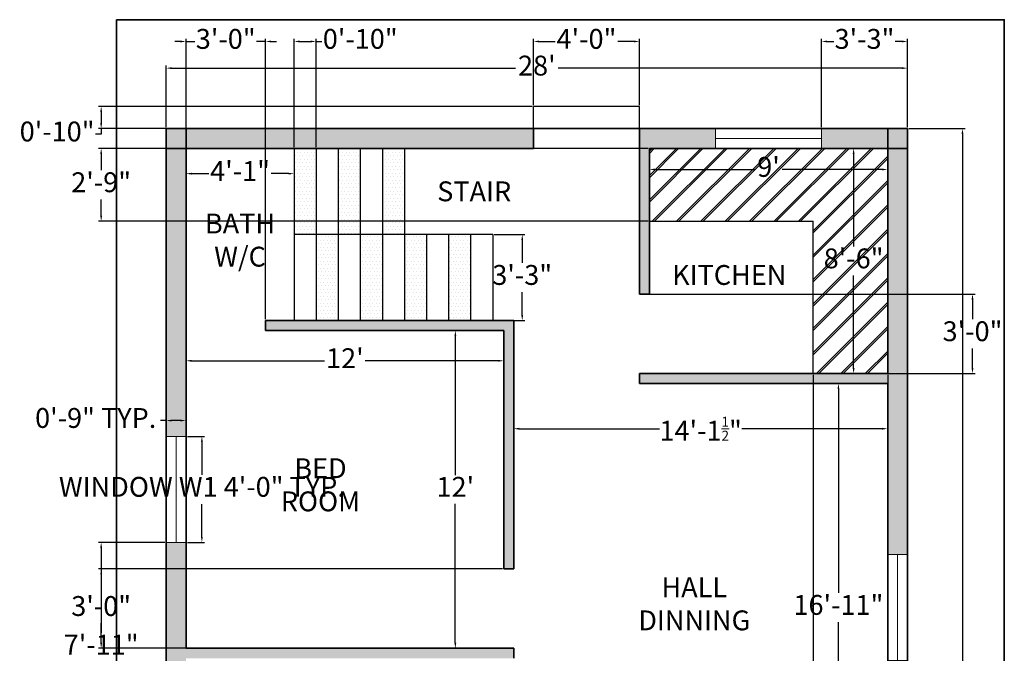
# Model space of a CAD drawing. Units: inches. Extents: x 4987 to 5457, y 8145 to 8785.
# Tile 3 of 3: x 4987 to 5434, y 8498 to 8785. Entities that reach past the tile are written whole.
import ezdxf

# ---------------------------------------------------------------- set-up
doc = ezdxf.new("R2010")
doc.units = ezdxf.units.IN
for name, color, linetype, lineweight in [('A-ANNO-DIMS', 2, 'Continuous', 18), ('A-ANNO-TTLB', 7, 'Continuous', 35), ('A-AREA-IDEN', 240, 'Continuous', 25), ('A-COLS', 7, 'Continuous', 35), ('A-COLS-PATT', 7, 'Continuous', 13), ('A-FLOR-FIXT', 8, 'Continuous', 25), ('A-FLOR-PATT', 8, 'Continuous', 13), ('A-FLOR-STRS', 7, 'Continuous', 25), ('A-GLAZ', 4, 'Continuous', 18), ('A-WALL', 7, 'Continuous', 35)]:
    doc.layers.add(name, color=color, linetype=linetype, lineweight=lineweight)
doc.layers.add('A-FIXT-PATT', color=67, linetype='Continuous', lineweight=13, true_color=0x727430)
doc.layers.add('A-WALL-PATT', color=67, linetype='Continuous', lineweight=13, true_color=0x727430)
doc.styles.get("Standard").update_dxf_attribs({"font": 'arial.ttf'})
doc.dimstyles.new('ISO-25', dxfattribs={"dimtxt": 9, "dimasz": 2.5, "dimexe": 1.25, "dimexo": 0.625, "dimgap": 2, "dimtad": 0, "dimtih": 1, "dimtoh": 1, "dimdec": 1, "dimlunit": 4, "dimtxsty": 'Standard', "dimcen": 2.5, "dimadec": 0, "dimazin": 0, "dimtfac": 0.5, "dimtdec": 1, "dimtmove": 0, "dimatfit": 3, "dimfxl": 1, "dimarcsym": 0})

# ---------------------------------------------------------------- blocks, each defined once
blk = doc.blocks.new('*D1')
at = {"layer": 'A-ANNO-DIMS', "color": 0, "lineweight": -2, "transparency": 16777216}
for p, q in [((5272.84, 8717.82), (5272.84, 8718.44)), ((5275.34, 8717.19), (5320.7, 8717.19)), ((5378.34, 8717.19), (5332.98, 8717.19)), ((5380.84, 8717.82), (5380.84, 8718.44))]:
    blk.add_line(p, q, dxfattribs=at)
at = {"layer": 'A-ANNO-DIMS', "color": 0, "transparency": 16777216}
for points in [[(5275.34, 8717.61), (5275.34, 8716.78), (5272.84, 8717.19)], [(5378.34, 8717.61), (5378.34, 8716.78), (5380.84, 8717.19)]]:
    blk.add_solid(points, dxfattribs=at)
at = {"layer": 'Defpoints', "color": 0, "transparency": 16777216}
for p in [(5272.84, 8717.19), (5380.84, 8717.19), (5380.84, 8717.19)]:
    blk.add_point(p, dxfattribs=at)
at = {"layer": 'A-ANNO-DIMS', "color": 0, "transparency": 16777216, "insert": (5326.84, 8717.19), "char_height": 9, "attachment_point": 5}
blk.add_mtext("9'", dxfattribs=at)
blk = doc.blocks.new('*D2')
at = {"layer": 'A-ANNO-DIMS', "color": 0, "lineweight": -2, "transparency": 16777216}
for p, q in [((5380.22, 8726.74), (5364.15, 8726.74)), ((5365.4, 8724.24), (5365.4, 8682.33)), ((5365.4, 8627.24), (5365.4, 8669.14)), ((5380.22, 8624.74), (5364.15, 8624.74))]:
    blk.add_line(p, q, dxfattribs=at)
at = {"layer": 'A-ANNO-DIMS', "color": 0, "transparency": 16777216}
for points in [[(5364.99, 8724.24), (5365.82, 8724.24), (5365.4, 8726.74)], [(5364.99, 8627.24), (5365.82, 8627.24), (5365.4, 8624.74)]]:
    blk.add_solid(points, dxfattribs=at)
at = {"layer": 'Defpoints', "color": 0, "transparency": 16777216}
for p in [(5365.4, 8726.74), (5380.84, 8726.74), (5380.84, 8624.74)]:
    blk.add_point(p, dxfattribs=at)
at = {"layer": 'A-ANNO-DIMS', "color": 0, "transparency": 16777216, "insert": (5365.4, 8675.74), "char_height": 9, "attachment_point": 5}
blk.add_mtext('8\'-6"', dxfattribs=at)
blk = doc.blocks.new('*D3')
at = {"layer": 'A-ANNO-DIMS', "color": 0, "lineweight": -2, "transparency": 16777216}
for p, q in [((5380.22, 8620.24), (5357.27, 8620.24)), ((5358.52, 8617.74), (5358.52, 8525.33)), ((5358.52, 8419.74), (5358.52, 8512.14)), ((5380.22, 8417.24), (5357.27, 8417.24))]:
    blk.add_line(p, q, dxfattribs=at)
at = {"layer": 'A-ANNO-DIMS', "color": 0, "transparency": 16777216}
for points in [[(5358.11, 8617.74), (5358.94, 8617.74), (5358.52, 8620.24)], [(5358.11, 8419.74), (5358.94, 8419.74), (5358.52, 8417.24)]]:
    blk.add_solid(points, dxfattribs=at)
at = {"layer": 'Defpoints', "color": 0, "transparency": 16777216}
for p in [(5380.84, 8620.24), (5358.52, 8417.24), (5380.84, 8417.24)]:
    blk.add_point(p, dxfattribs=at)
at = {"layer": 'A-ANNO-DIMS', "color": 0, "transparency": 16777216, "insert": (5358.52, 8518.74), "char_height": 9, "attachment_point": 5}
blk.add_mtext('16\'-11"', dxfattribs=at)
blk = doc.blocks.new('*D4')
at = {"layer": 'A-ANNO-DIMS', "color": 0, "lineweight": -2, "transparency": 16777216}
for p, q in [((5211.34, 8619.61), (5211.34, 8598.5)), ((5380.84, 8619.61), (5380.84, 8598.5)), ((5213.84, 8599.75), (5277.41, 8599.75)), ((5378.34, 8599.75), (5314.77, 8599.75))]:
    blk.add_line(p, q, dxfattribs=at)
at = {"layer": 'A-ANNO-DIMS', "color": 0, "transparency": 16777216}
for points in [[(5213.84, 8600.16), (5213.84, 8599.33), (5211.34, 8599.75)], [(5378.34, 8600.16), (5378.34, 8599.33), (5380.84, 8599.75)]]:
    blk.add_solid(points, dxfattribs=at)
at = {"layer": 'Defpoints', "color": 0, "transparency": 16777216}
for p in [(5211.34, 8620.24), (5380.84, 8620.24), (5211.34, 8599.75)]:
    blk.add_point(p, dxfattribs=at)
at = {"layer": 'A-ANNO-DIMS', "color": 0, "transparency": 16777216, "insert": (5296.09, 8599.75), "char_height": 9, "attachment_point": 5}
blk.add_mtext('14\'-1{\\H0.5x;\\S1/2;}"', dxfattribs=at)
blk = doc.blocks.new('*D5')
at = {"layer": 'A-ANNO-DIMS', "color": 0, "lineweight": -2, "transparency": 16777216}
for p, q in [((5202.47, 8687.74), (5216.47, 8687.74)), ((5215.22, 8685.24), (5215.22, 8674.83)), ((5215.22, 8651.24), (5215.22, 8661.64)), ((5202.47, 8648.74), (5216.47, 8648.74))]:
    blk.add_line(p, q, dxfattribs=at)
at = {"layer": 'A-ANNO-DIMS', "color": 0, "transparency": 16777216}
for points in [[(5214.8, 8685.24), (5215.64, 8685.24), (5215.22, 8687.74)], [(5214.8, 8651.24), (5215.64, 8651.24), (5215.22, 8648.74)]]:
    blk.add_solid(points, dxfattribs=at)
at = {"layer": 'Defpoints', "color": 0, "transparency": 16777216}
for p in [(5201.84, 8687.74), (5215.22, 8687.74), (5201.84, 8648.74)]:
    blk.add_point(p, dxfattribs=at)
at = {"layer": 'A-ANNO-DIMS', "color": 0, "transparency": 16777216, "insert": (5215.22, 8668.24), "char_height": 9, "attachment_point": 5}
blk.add_mtext('3\'-3"', dxfattribs=at)
blk = doc.blocks.new('*D6')
at = {"layer": 'A-ANNO-DIMS', "color": 0, "lineweight": -2, "transparency": 16777216}
for p, q in [((5062.84, 8726.11), (5062.84, 8714.05)), ((5111.84, 8726.11), (5111.84, 8714.05)), ((5065.34, 8715.3), (5073.2, 8715.3)), ((5109.34, 8715.3), (5101.48, 8715.3))]:
    blk.add_line(p, q, dxfattribs=at)
at = {"layer": 'A-ANNO-DIMS', "color": 0, "transparency": 16777216}
for points in [[(5065.34, 8715.71), (5065.34, 8714.88), (5062.84, 8715.3)], [(5109.34, 8715.71), (5109.34, 8714.88), (5111.84, 8715.3)]]:
    blk.add_solid(points, dxfattribs=at)
at = {"layer": 'Defpoints', "color": 0, "transparency": 16777216}
for p in [(5062.84, 8726.74), (5111.84, 8726.74), (5062.84, 8715.3)]:
    blk.add_point(p, dxfattribs=at)
at = {"layer": 'A-ANNO-DIMS', "color": 0, "transparency": 16777216, "insert": (5087.34, 8715.3), "char_height": 9, "attachment_point": 5}
blk.add_mtext('4\'-1"', dxfattribs=at)
blk = doc.blocks.new('*D7')
at = {"layer": 'A-ANNO-DIMS', "color": 0, "lineweight": -2, "transparency": 16777216}
for p, q in [((5062.84, 8643.61), (5062.84, 8629.26)), ((5206.84, 8643.61), (5206.84, 8629.26)), ((5065.34, 8630.51), (5125.63, 8630.51)), ((5204.34, 8630.51), (5144.05, 8630.51))]:
    blk.add_line(p, q, dxfattribs=at)
at = {"layer": 'A-ANNO-DIMS', "color": 0, "transparency": 16777216}
for points in [[(5065.34, 8630.93), (5065.34, 8630.1), (5062.84, 8630.51)], [(5204.34, 8630.93), (5204.34, 8630.1), (5206.84, 8630.51)]]:
    blk.add_solid(points, dxfattribs=at)
at = {"layer": 'Defpoints', "color": 0, "transparency": 16777216}
for p in [(5062.84, 8644.24), (5206.84, 8644.24), (5062.84, 8630.51)]:
    blk.add_point(p, dxfattribs=at)
at = {"layer": 'A-ANNO-DIMS', "color": 0, "transparency": 16777216, "insert": (5134.84, 8630.51), "char_height": 9, "attachment_point": 5}
blk.add_mtext("12'", dxfattribs=at)
blk = doc.blocks.new('*D8')
at = {"layer": 'A-ANNO-DIMS', "color": 0, "lineweight": -2, "transparency": 16777216}
for p, q in [((5185.53, 8644.24), (5186.15, 8644.24)), ((5184.9, 8641.74), (5184.9, 8578.75)), ((5184.9, 8502.74), (5184.9, 8565.72)), ((5185.53, 8500.24), (5186.15, 8500.24))]:
    blk.add_line(p, q, dxfattribs=at)
at = {"layer": 'A-ANNO-DIMS', "color": 0, "transparency": 16777216}
for points in [[(5184.49, 8641.74), (5185.32, 8641.74), (5184.9, 8644.24)], [(5184.49, 8502.74), (5185.32, 8502.74), (5184.9, 8500.24)]]:
    blk.add_solid(points, dxfattribs=at)
at = {"layer": 'Defpoints', "color": 0, "transparency": 16777216}
for p in [(5184.9, 8644.24), (5184.9, 8644.24), (5184.9, 8500.24)]:
    blk.add_point(p, dxfattribs=at)
at = {"layer": 'A-ANNO-DIMS', "color": 0, "transparency": 16777216, "insert": (5184.9, 8572.24), "char_height": 9, "attachment_point": 5}
blk.add_mtext("12'", dxfattribs=at)
blk = doc.blocks.new('*D19')
at = {"layer": 'A-ANNO-DIMS', "color": 0, "lineweight": -2, "transparency": 16777216}
for p, q in [((5390.47, 8735.74), (5415.98, 8735.74)), ((5414.73, 8733.24), (5414.73, 8478.24)), ((5414.73, 8210.24), (5414.73, 8465.24)), ((5390.47, 8207.74), (5415.98, 8207.74))]:
    blk.add_line(p, q, dxfattribs=at)
at = {"layer": 'A-ANNO-DIMS', "color": 0, "transparency": 16777216}
for points in [[(5414.31, 8733.24), (5415.15, 8733.24), (5414.73, 8735.74)], [(5414.31, 8210.24), (5415.15, 8210.24), (5414.73, 8207.74)]]:
    blk.add_solid(points, dxfattribs=at)
at = {"layer": 'Defpoints', "color": 0, "transparency": 16777216}
for p in [(5389.84, 8735.74), (5389.84, 8207.74), (5414.73, 8207.74)]:
    blk.add_point(p, dxfattribs=at)
at = {"layer": 'A-ANNO-DIMS', "color": 0, "transparency": 16777216, "insert": (5414.73, 8471.74), "char_height": 9, "attachment_point": 5}
blk.add_mtext("44'", dxfattribs=at)
blk = doc.blocks.new('*D20')
at = {"layer": 'A-ANNO-DIMS', "color": 0, "lineweight": -2, "transparency": 16777216}
for p, q in [((5053.84, 8736.36), (5053.84, 8764.35)), ((5389.84, 8736.36), (5389.84, 8764.35)), ((5056.34, 8763.1), (5212.13, 8763.1)), ((5387.34, 8763.1), (5231.55, 8763.1))]:
    blk.add_line(p, q, dxfattribs=at)
at = {"layer": 'A-ANNO-DIMS', "color": 0, "transparency": 16777216}
for points in [[(5056.34, 8763.52), (5056.34, 8762.68), (5053.84, 8763.1)], [(5387.34, 8763.52), (5387.34, 8762.68), (5389.84, 8763.1)]]:
    blk.add_solid(points, dxfattribs=at)
at = {"layer": 'Defpoints', "color": 0, "transparency": 16777216}
for p in [(5389.84, 8763.1), (5053.84, 8735.74), (5389.84, 8735.74)]:
    blk.add_point(p, dxfattribs=at)
at = {"layer": 'A-ANNO-DIMS', "color": 0, "transparency": 16777216, "insert": (5221.84, 8763.1), "char_height": 9, "attachment_point": 5}
blk.add_mtext("28'", dxfattribs=at)
blk = doc.blocks.new('WIN-48IN')
for p, q in [((0, 0), (0, 9)), ((48, 0), (48, 9)), ((0, 4.5), (48, 4.5))]:
    blk.add_line(p, q)
blk = doc.blocks.new('COL-CORNER-9IN')
for q in [(0, 0), (9, 9)]:
    blk.add_line((0, 9), q)
blk = doc.blocks.new('*D24')
at = {"layer": 'A-ANNO-DIMS', "color": 0, "lineweight": -2, "transparency": 16777216}
for p, q in [((5063.47, 8596.24), (5071.29, 8596.24)), ((5070.04, 8593.74), (5070.04, 8578.89)), ((5070.04, 8550.74), (5070.04, 8565.58)), ((5063.47, 8548.24), (5071.29, 8548.24))]:
    blk.add_line(p, q, dxfattribs=at)
at = {"layer": 'A-ANNO-DIMS', "color": 0, "transparency": 16777216}
for points in [[(5069.62, 8593.74), (5070.46, 8593.74), (5070.04, 8596.24)], [(5069.62, 8550.74), (5070.46, 8550.74), (5070.04, 8548.24)]]:
    blk.add_solid(points, dxfattribs=at)
at = {"layer": 'Defpoints', "color": 0, "transparency": 16777216}
for p in [(5062.84, 8596.24), (5070.04, 8596.24), (5062.84, 8548.24)]:
    blk.add_point(p, dxfattribs=at)
at = {"layer": 'A-ANNO-DIMS', "color": 0, "transparency": 16777216, "insert": (5070.04, 8572.24), "char_height": 9, "attachment_point": 5}
blk.add_mtext('WINDOW W1 4\'-0" TYP.', dxfattribs=at)
blk = doc.blocks.new('*D25')
at = {"layer": 'A-ANNO-DIMS', "color": 0, "lineweight": -2, "transparency": 16777216}
for p, q in [((5053.84, 8596.86), (5053.84, 8604.69)), ((5062.84, 8596.86), (5062.84, 8604.69)), ((5053.84, 8603.44), (5051.34, 8603.44)), ((5060.34, 8603.44), (5056.34, 8603.44))]:
    blk.add_line(p, q, dxfattribs=at)
at = {"layer": 'A-ANNO-DIMS', "color": 0, "transparency": 16777216}
for points in [[(5056.34, 8603.85), (5056.34, 8603.02), (5053.84, 8603.44)], [(5060.34, 8603.85), (5060.34, 8603.02), (5062.84, 8603.44)]]:
    blk.add_solid(points, dxfattribs=at)
at = {"layer": 'Defpoints', "color": 0, "transparency": 16777216}
for p in [(5053.84, 8603.44), (5053.84, 8596.24), (5062.84, 8596.24)]:
    blk.add_point(p, dxfattribs=at)
at = {"layer": 'A-ANNO-DIMS', "color": 0, "transparency": 16777216, "insert": (5021.91, 8603.44), "char_height": 9, "attachment_point": 5}
blk.add_mtext('0\'-9" TYP.', dxfattribs=at)
blk = doc.blocks.new('*D32')
at = {"layer": 'A-ANNO-DIMS', "color": 0, "lineweight": -2, "transparency": 16777216}
for p, q in [((5053.22, 8548.24), (5023.14, 8548.24)), ((5024.39, 8545.74), (5024.39, 8507.25)), ((5024.39, 8455.74), (5024.39, 8494.22)), ((5053.22, 8453.24), (5023.14, 8453.24))]:
    blk.add_line(p, q, dxfattribs=at)
at = {"layer": 'A-ANNO-DIMS', "color": 0, "transparency": 16777216}
for points in [[(5023.97, 8545.74), (5024.81, 8545.74), (5024.39, 8548.24)], [(5023.97, 8455.74), (5024.81, 8455.74), (5024.39, 8453.24)]]:
    blk.add_solid(points, dxfattribs=at)
at = {"layer": 'Defpoints', "color": 0, "transparency": 16777216}
for p in [(5024.39, 8548.24), (5053.84, 8548.24), (5053.84, 8453.24)]:
    blk.add_point(p, dxfattribs=at)
at = {"layer": 'A-ANNO-DIMS', "color": 0, "transparency": 16777216, "insert": (5024.39, 8500.74), "char_height": 9, "attachment_point": 5}
blk.add_mtext('7\'-11"', dxfattribs=at)
blk = doc.blocks.new('*D36')
at = {"layer": 'A-ANNO-DIMS', "color": 0, "lineweight": -2, "transparency": 16777216}
for p, q in [((5350.84, 8736.36), (5350.84, 8776.44)), ((5353.34, 8775.19), (5356.38, 8775.19)), ((5387.34, 8775.19), (5384.3, 8775.19)), ((5389.84, 8736.36), (5389.84, 8776.44))]:
    blk.add_line(p, q, dxfattribs=at)
at = {"layer": 'A-ANNO-DIMS', "color": 0, "transparency": 16777216}
for points in [[(5353.34, 8775.6), (5353.34, 8774.77), (5350.84, 8775.19)], [(5387.34, 8775.6), (5387.34, 8774.77), (5389.84, 8775.19)]]:
    blk.add_solid(points, dxfattribs=at)
at = {"layer": 'Defpoints', "color": 0, "transparency": 16777216}
for p in [(5389.84, 8775.19), (5350.84, 8735.74), (5389.84, 8735.74)]:
    blk.add_point(p, dxfattribs=at)
at = {"layer": 'A-ANNO-DIMS', "color": 0, "transparency": 16777216, "insert": (5370.34, 8775.19), "char_height": 9, "attachment_point": 5}
blk.add_mtext('3\'-3"', dxfattribs=at)
blk = doc.blocks.new('*D39')
at = {"layer": 'A-ANNO-DIMS', "color": 0, "lineweight": -2, "transparency": 16777216}
for p, q in [((5220.34, 8746.36), (5220.34, 8776.44)), ((5222.84, 8775.19), (5230.2, 8775.19)), ((5265.84, 8775.19), (5258.48, 8775.19)), ((5268.34, 8746.36), (5268.34, 8776.44))]:
    blk.add_line(p, q, dxfattribs=at)
at = {"layer": 'A-ANNO-DIMS', "color": 0, "transparency": 16777216}
for points in [[(5222.84, 8775.6), (5222.84, 8774.77), (5220.34, 8775.19)], [(5265.84, 8775.6), (5265.84, 8774.77), (5268.34, 8775.19)]]:
    blk.add_solid(points, dxfattribs=at)
at = {"layer": 'Defpoints', "color": 0, "transparency": 16777216}
for p in [(5268.34, 8775.19), (5220.34, 8745.74), (5268.34, 8745.74)]:
    blk.add_point(p, dxfattribs=at)
at = {"layer": 'A-ANNO-DIMS', "color": 0, "transparency": 16777216, "insert": (5244.34, 8775.19), "char_height": 9, "attachment_point": 5}
blk.add_mtext('4\'-0"', dxfattribs=at)
blk = doc.blocks.new('*D40')
at = {"layer": 'A-ANNO-DIMS', "color": 0, "lineweight": -2, "transparency": 16777216}
for p, q in [((5219.72, 8745.74), (5023.14, 8745.74)), ((5024.39, 8743.24), (5024.39, 8738.24)), ((5024.39, 8733.24), (5021.89, 8733.24)), ((5219.72, 8735.74), (5023.14, 8735.74)), ((5024.39, 8735.74), (5024.39, 8733.24))]:
    blk.add_line(p, q, dxfattribs=at)
at = {"layer": 'A-ANNO-DIMS', "color": 0, "transparency": 16777216}
for points in [[(5023.97, 8743.24), (5024.81, 8743.24), (5024.39, 8745.74)], [(5023.97, 8738.24), (5024.81, 8738.24), (5024.39, 8735.74)]]:
    blk.add_solid(points, dxfattribs=at)
at = {"layer": 'Defpoints', "color": 0, "transparency": 16777216}
for p in [(5220.34, 8745.74), (5024.39, 8735.74), (5220.34, 8735.74)]:
    blk.add_point(p, dxfattribs=at)
at = {"layer": 'A-ANNO-DIMS', "color": 0, "transparency": 16777216, "insert": (5004.43, 8733.24), "char_height": 9, "attachment_point": 5}
blk.add_mtext('0\'-10"', dxfattribs=at)
blk = doc.blocks.new('*D41')
at = {"layer": 'A-ANNO-DIMS', "color": 0, "lineweight": -2, "transparency": 16777216}
for p, q in [((5111.84, 8727.36), (5111.84, 8776.44)), ((5114.34, 8775.19), (5119.34, 8775.19)), ((5121.84, 8727.36), (5121.84, 8776.44)), ((5121.84, 8775.19), (5124.34, 8775.19))]:
    blk.add_line(p, q, dxfattribs=at)
at = {"layer": 'A-ANNO-DIMS', "color": 0, "transparency": 16777216}
for points in [[(5114.34, 8775.6), (5114.34, 8774.77), (5111.84, 8775.19)], [(5119.34, 8775.6), (5119.34, 8774.77), (5121.84, 8775.19)]]:
    blk.add_solid(points, dxfattribs=at)
at = {"layer": 'Defpoints', "color": 0, "transparency": 16777216}
for p in [(5121.84, 8775.19), (5111.84, 8726.74), (5121.84, 8726.74)]:
    blk.add_point(p, dxfattribs=at)
at = {"layer": 'A-ANNO-DIMS', "color": 0, "transparency": 16777216, "insert": (5141.8, 8775.19), "char_height": 9, "attachment_point": 5}
blk.add_mtext('0\'-10"', dxfattribs=at)
blk = doc.blocks.new('*D42')
at = {"layer": 'A-ANNO-DIMS', "color": 0, "lineweight": -2, "transparency": 16777216}
for p, q in [((5347.07, 8624.11), (5347.07, 8157.04)), ((5380.84, 8624.11), (5380.84, 8157.04)), ((5349.57, 8158.29), (5378.34, 8158.29)), ((5380.84, 8158.29), (5383.34, 8158.29))]:
    blk.add_line(p, q, dxfattribs=at)
at = {"layer": 'A-ANNO-DIMS', "color": 0, "transparency": 16777216}
for points in [[(5349.57, 8158.7), (5349.57, 8157.87), (5347.07, 8158.29)], [(5378.34, 8158.7), (5378.34, 8157.87), (5380.84, 8158.29)]]:
    blk.add_solid(points, dxfattribs=at)
at = {"layer": 'Defpoints', "color": 0, "transparency": 16777216}
for p in [(5347.07, 8624.74), (5380.84, 8624.74), (5380.84, 8158.29)]:
    blk.add_point(p, dxfattribs=at)
at = {"layer": 'A-ANNO-DIMS', "color": 0, "transparency": 16777216, "insert": (5400.88, 8158.29), "char_height": 9, "attachment_point": 5}
blk.add_mtext('2\'-10"', dxfattribs=at)
blk = doc.blocks.new('*D43')
at = {"layer": 'A-ANNO-DIMS', "color": 0, "lineweight": -2, "transparency": 16777216}
for p, q in [((5272.22, 8726.74), (5023.14, 8726.74)), ((5024.39, 8724.24), (5024.39, 8716.83)), ((5024.39, 8696.24), (5024.39, 8703.64)), ((5272.22, 8693.74), (5023.14, 8693.74))]:
    blk.add_line(p, q, dxfattribs=at)
at = {"layer": 'A-ANNO-DIMS', "color": 0, "transparency": 16777216}
for points in [[(5023.97, 8724.24), (5024.81, 8724.24), (5024.39, 8726.74)], [(5023.97, 8696.24), (5024.81, 8696.24), (5024.39, 8693.74)]]:
    blk.add_solid(points, dxfattribs=at)
at = {"layer": 'Defpoints', "color": 0, "transparency": 16777216}
for p in [(5024.39, 8726.74), (5272.84, 8726.74), (5272.84, 8693.74)]:
    blk.add_point(p, dxfattribs=at)
at = {"layer": 'A-ANNO-DIMS', "color": 0, "transparency": 16777216, "insert": (5024.39, 8710.24), "char_height": 9, "attachment_point": 5}
blk.add_mtext('2\'-9"', dxfattribs=at)
blk = doc.blocks.new('*D44')
at = {"layer": 'A-ANNO-DIMS', "color": 0, "lineweight": -2, "transparency": 16777216}
for p, q in [((5268.97, 8660.74), (5420.54, 8660.74)), ((5419.29, 8658.24), (5419.29, 8649.33)), ((5419.29, 8627.24), (5419.29, 8636.14)), ((5268.97, 8624.74), (5420.54, 8624.74))]:
    blk.add_line(p, q, dxfattribs=at)
at = {"layer": 'A-ANNO-DIMS', "color": 0, "transparency": 16777216}
for points in [[(5418.87, 8658.24), (5419.71, 8658.24), (5419.29, 8660.74)], [(5418.87, 8627.24), (5419.71, 8627.24), (5419.29, 8624.74)]]:
    blk.add_solid(points, dxfattribs=at)
at = {"layer": 'Defpoints', "color": 0, "transparency": 16777216}
for p in [(5268.34, 8660.74), (5419.29, 8660.74), (5268.34, 8624.74)]:
    blk.add_point(p, dxfattribs=at)
at = {"layer": 'A-ANNO-DIMS', "color": 0, "transparency": 16777216, "insert": (5419.29, 8642.74), "char_height": 9, "attachment_point": 5}
blk.add_mtext('3\'-0"', dxfattribs=at)
blk = doc.blocks.new('*D45')
at = {"layer": 'A-ANNO-DIMS', "color": 0, "lineweight": -2, "transparency": 16777216}
for p, q in [((5206.22, 8536.24), (5023.14, 8536.24)), ((5024.39, 8533.74), (5024.39, 8524.83)), ((5024.39, 8502.74), (5024.39, 8511.64)), ((5206.22, 8500.24), (5023.14, 8500.24))]:
    blk.add_line(p, q, dxfattribs=at)
at = {"layer": 'A-ANNO-DIMS', "color": 0, "transparency": 16777216}
for points in [[(5023.97, 8533.74), (5024.81, 8533.74), (5024.39, 8536.24)], [(5023.97, 8502.74), (5024.81, 8502.74), (5024.39, 8500.24)]]:
    blk.add_solid(points, dxfattribs=at)
at = {"layer": 'Defpoints', "color": 0, "transparency": 16777216}
for p in [(5024.39, 8536.24), (5206.84, 8536.24), (5206.84, 8500.24)]:
    blk.add_point(p, dxfattribs=at)
at = {"layer": 'A-ANNO-DIMS', "color": 0, "transparency": 16777216, "insert": (5024.39, 8518.24), "char_height": 9, "attachment_point": 5}
blk.add_mtext('3\'-0"', dxfattribs=at)
blk = doc.blocks.new('*D50')
at = {"layer": 'A-ANNO-DIMS', "color": 0, "lineweight": -2, "transparency": 16777216}
for p, q in [((5060.34, 8775.19), (5057.84, 8775.19)), ((5062.84, 8649.36), (5062.84, 8776.44)), ((5062.84, 8775.19), (5066.88, 8775.19)), ((5098.84, 8775.19), (5094.8, 8775.19)), ((5098.84, 8649.36), (5098.84, 8776.44)), ((5101.34, 8775.19), (5103.84, 8775.19))]:
    blk.add_line(p, q, dxfattribs=at)
at = {"layer": 'A-ANNO-DIMS', "color": 0, "transparency": 16777216}
for points in [[(5060.34, 8775.6), (5060.34, 8774.77), (5062.84, 8775.19)], [(5101.34, 8775.6), (5101.34, 8774.77), (5098.84, 8775.19)]]:
    blk.add_solid(points, dxfattribs=at)
at = {"layer": 'Defpoints', "color": 0, "transparency": 16777216}
for p in [(5098.84, 8775.19), (5062.84, 8648.74), (5098.84, 8648.74)]:
    blk.add_point(p, dxfattribs=at)
at = {"layer": 'A-ANNO-DIMS', "color": 0, "transparency": 16777216, "insert": (5080.84, 8775.19), "char_height": 9, "attachment_point": 5}
blk.add_mtext('3\'-0"', dxfattribs=at)

msp = doc.modelspace()

# ---------------------------------------------------------------- hatches: boundary and pattern name
at = {"layer": 'A-COLS-PATT'}
h = msp.add_hatch(color=256, dxfattribs=at)
h.dxf.hatch_style = 1
h.paths.add_polyline_path([(5062.84, 8735.74), (5053.84, 8735.74), (5053.84, 8726.74), (5062.84, 8726.74)])
h.paths.add_polyline_path([(5389.84, 8735.74), (5380.84, 8735.74), (5380.84, 8726.74), (5389.84, 8726.74)])
h.paths.add_polyline_path([(5389.84, 8216.74), (5380.84, 8216.74), (5380.84, 8207.74), (5389.84, 8207.74)])
h.paths.add_polyline_path([(5062.84, 8216.74), (5053.84, 8216.74), (5053.84, 8207.74), (5062.84, 8207.74)])
at = {"layer": 'A-FIXT-PATT'}
h = msp.add_hatch(dxfattribs=at)
h.set_pattern_fill('JIS_LC_8A', color=256)
h.paths.add_polyline_path([(5380.84, 8726.74), (5272.84, 8726.74), (5272.84, 8693.74), (5347.07, 8693.74), (5347.07, 8624.74), (5380.84, 8624.74)])
at = {"layer": 'A-FLOR-PATT'}
h = msp.add_hatch(dxfattribs=at)
h.set_pattern_fill('DOTS', color=256)
h.paths.add_polyline_path([(5121.84, 8726.74), (5111.84, 8726.74), (5111.84, 8687.74), (5121.84, 8687.74)])
h.paths.add_polyline_path([(5141.84, 8726.74), (5131.84, 8726.74), (5131.84, 8687.74), (5141.84, 8687.74)])
h.paths.add_polyline_path([(5161.84, 8726.74), (5151.84, 8726.74), (5151.84, 8687.74), (5161.84, 8687.74)])
h.paths.add_polyline_path([(5131.84, 8687.74), (5121.84, 8687.74), (5121.84, 8648.74), (5131.84, 8648.74)])
h.paths.add_polyline_path([(5151.84, 8687.74), (5141.84, 8687.74), (5141.84, 8648.74), (5151.84, 8648.74)])
h.paths.add_polyline_path([(5171.84, 8687.74), (5161.84, 8687.74), (5161.84, 8648.74), (5171.84, 8648.74)])
h.paths.add_polyline_path([(5191.84, 8687.74), (5181.84, 8687.74), (5181.84, 8648.74), (5191.84, 8648.74)])
at = {"layer": 'A-WALL-PATT'}
h = msp.add_hatch(color=256, dxfattribs=at)
h.dxf.hatch_style = 1
h.paths.add_polyline_path([(5220.34, 8735.74), (5062.84, 8735.74), (5062.84, 8726.74), (5111.84, 8726.74), (5220.34, 8726.74)])
h.paths.add_polyline_path([(5062.84, 8548.24), (5053.84, 8548.24), (5053.84, 8453.24), (5062.84, 8453.24), (5062.84, 8495.74), (5206.84, 8495.74), (5211.34, 8495.74), (5211.34, 8500.24), (5206.84, 8500.24), (5062.84, 8500.24)])
h.paths.add_polyline_path([(5211.34, 8362.74), (5211.34, 8412.74), (5211.34, 8417.24), (5211.34, 8459.74), (5206.84, 8459.74), (5206.84, 8417.24), (5206.84, 8412.74), (5206.84, 8362.74), (5062.84, 8362.74), (5062.84, 8405.24), (5053.84, 8405.24), (5053.84, 8311.49), (5062.84, 8311.49), (5062.84, 8358.24), (5206.84, 8358.24), (5211.34, 8358.24)])
h.paths.add_polyline_path([(5062.84, 8263.49), (5053.84, 8263.49), (5053.84, 8216.74), (5062.84, 8216.74)])
h.paths.add_polyline_path([(5211.34, 8216.74), (5206.84, 8216.74), (5062.84, 8216.74), (5062.84, 8207.74), (5211.34, 8207.74)])
h.paths.add_polyline_path([(5380.84, 8216.74), (5271.34, 8216.74), (5271.34, 8207.74), (5380.84, 8207.74)])
h.paths.add_polyline_path([(5389.84, 8314.24), (5380.84, 8314.24), (5380.84, 8305.24), (5332.84, 8305.24), (5332.84, 8311.24), (5328.34, 8311.24), (5328.34, 8305.24), (5247.34, 8305.24), (5247.34, 8300.74), (5380.84, 8300.74), (5380.84, 8216.74), (5389.84, 8216.74)])
h.paths.add_polyline_path([(5389.84, 8370.24), (5380.84, 8370.24), (5380.84, 8351.74), (5328.34, 8351.74), (5320.84, 8351.74), (5320.84, 8347.24), (5328.34, 8347.24), (5332.84, 8347.24), (5380.84, 8347.24), (5380.84, 8338.24), (5389.84, 8338.24)])
h.paths.add_polyline_path([(5389.84, 8494.74), (5380.84, 8494.74), (5380.84, 8417.24), (5280.34, 8417.24), (5280.34, 8412.74), (5280.34, 8351.74), (5280.34, 8347.24), (5284.84, 8347.24), (5284.84, 8351.74), (5284.84, 8412.74), (5328.34, 8412.74), (5380.84, 8412.74), (5380.84, 8394.24), (5389.84, 8394.24)])
h.paths.add_polyline_path([(5389.84, 8726.74), (5380.84, 8726.74), (5380.84, 8624.74), (5272.84, 8624.74), (5268.34, 8624.74), (5268.34, 8620.24), (5380.84, 8620.24), (5380.84, 8542.74), (5389.84, 8542.74)])
h.paths.add_polyline_path([(5062.84, 8726.74), (5053.84, 8726.74), (5053.84, 8596.24), (5062.84, 8596.24), (5062.84, 8644.24), (5062.84, 8648.74)])
h.paths.add_polyline_path([(5302.84, 8735.74), (5268.34, 8735.74), (5268.34, 8726.74), (5268.34, 8660.74), (5272.84, 8660.74), (5272.84, 8726.74), (5302.84, 8726.74)])
h.paths.add_polyline_path([(5380.84, 8735.74), (5350.84, 8735.74), (5350.84, 8726.74), (5380.84, 8726.74)])
h.paths.add_polyline_path([(5211.34, 8648.74), (5206.84, 8648.74), (5098.84, 8648.74), (5098.84, 8644.24), (5206.84, 8644.24), (5206.84, 8624.74), (5206.84, 8536.24), (5211.34, 8536.24), (5211.34, 8620.24), (5211.34, 8624.74)])
h.paths.add_polyline_path([(5211.34, 8305.24), (5211.34, 8322.24), (5206.84, 8322.24), (5206.84, 8305.24), (5206.84, 8300.74), (5206.84, 8252.74), (5211.34, 8252.74), (5211.34, 8300.74)])

# ---------------------------------------------------------------- linework, layer by layer
at = {"layer": 'A-ANNO-TTLB'}
msp.add_lwpolyline([(5031.32, 8785.05), (5433.7, 8785.05), (5433.7, 8175.66), (5031.32, 8175.66)], close=True, dxfattribs=at)
at = {"layer": 'A-FLOR-FIXT'}
for p in [(5272.84, 8693.74), (5347.07, 8624.74)]:
    msp.add_line(p, (5347.07, 8693.74), dxfattribs=at)
at = {"layer": 'A-FLOR-STRS'}
for p, q in [((5220.34, 8735.74), (5220.34, 8745.74)), ((5268.34, 8745.74), (5220.34, 8745.74)), ((5268.34, 8735.74), (5268.34, 8745.74)), ((5111.84, 8726.74), (5111.84, 8648.74)), ((5121.84, 8726.74), (5121.84, 8648.74)), ((5131.84, 8726.74), (5131.84, 8648.74)), ((5141.84, 8726.74), (5141.84, 8648.74)), ((5151.84, 8726.74), (5151.84, 8648.74)), ((5161.84, 8726.74), (5161.84, 8648.74)), ((5201.84, 8687.74), (5111.84, 8687.74)), ((5171.84, 8687.74), (5171.84, 8648.74)), ((5181.84, 8687.74), (5181.84, 8648.74)), ((5191.84, 8687.74), (5191.84, 8648.74)), ((5201.84, 8687.74), (5201.84, 8648.74))]:
    msp.add_line(p, q, dxfattribs=at)
at = {"layer": 'A-WALL'}
for p, q in [((5053.84, 8735.74), (5389.84, 8735.74)), ((5053.84, 8207.74), (5053.84, 8735.74)), ((5220.34, 8726.74), (5220.34, 8735.74)), ((5268.34, 8726.74), (5268.34, 8735.74)), ((5389.84, 8735.74), (5389.84, 8207.74)), ((5062.84, 8726.74), (5220.34, 8726.74)), ((5062.84, 8648.74), (5062.84, 8726.74)), ((5062.84, 8726.74), (5111.84, 8726.74)), ((5268.34, 8726.74), (5268.34, 8660.74)), ((5272.84, 8726.74), (5272.84, 8660.74)), ((5272.84, 8726.74), (5380.84, 8726.74)), ((5380.84, 8726.74), (5380.84, 8624.74)), ((5272.84, 8660.74), (5268.34, 8660.74)), ((5062.84, 8648.74), (5062.84, 8644.24)), ((5206.84, 8648.74), (5098.84, 8648.74)), ((5098.84, 8648.74), (5098.84, 8644.24)), ((5206.84, 8648.74), (5211.34, 8648.74)), ((5211.34, 8624.74), (5211.34, 8648.74)), ((5062.84, 8500.24), (5062.84, 8644.24)), ((5206.84, 8644.24), (5098.84, 8644.24)), ((5206.84, 8644.24), (5206.84, 8624.74)), ((5206.84, 8624.74), (5206.84, 8536.24)), ((5211.34, 8624.74), (5211.34, 8620.24)), ((5268.34, 8624.74), (5268.34, 8620.24)), ((5272.84, 8624.74), (5268.34, 8624.74)), ((5380.84, 8624.74), (5272.84, 8624.74)), ((5211.34, 8620.24), (5211.34, 8536.24)), ((5380.84, 8620.24), (5268.34, 8620.24)), ((5380.84, 8620.24), (5380.84, 8417.24)), ((5206.84, 8536.24), (5211.34, 8536.24)), ((5206.84, 8500.24), (5062.84, 8500.24)), ((5206.84, 8500.24), (5211.34, 8500.24)), ((5211.34, 8500.24), (5211.34, 8495.74))]:
    msp.add_line(p, q, dxfattribs=at)

# ---------------------------------------------------------------- block references
at = {"layer": 'A-COLS'}
for p, rotation in [((5062.84, 8735.74), 180), ((5389.84, 8726.73), 89.9999999999884)]:
    msp.add_blockref('COL-CORNER-9IN', p, dxfattribs=dict(at, rotation=rotation))
at = {"layer": 'A-GLAZ'}
msp.add_blockref('WIN-48IN', (5302.84, 8726.74), dxfattribs=at)
for p, rotation in [((5062.84, 8548.23), 89.9999999999979), ((5389.84, 8494.73), 90.00000000000134)]:
    msp.add_blockref('WIN-48IN', p, dxfattribs=dict(at, rotation=rotation))

# ---------------------------------------------------------------- texts
at = {"layer": 'A-AREA-IDEN', "char_height": 9, "attachment_point": 1}
for s, width, insert in [('\\pxqc;{\\fArial|b1|i0|c0|p34;STAIR}', 59.0154, (5163.94, 8711.79)), ('\\pxqc;{\\fArial|b1|i0|c0|p34;BATH\\PW/C}', 39.1775, (5067.73, 8697.19)), ('\\pxqc;{\\fArial|b1|i0|c0|p34;KITCHEN}', 63.7916, (5277.13, 8673.9)), ('\\pxqc;{\\fArial|b1|i0|c0|p34;BED\\PROOM}', 79.9005, (5083.83, 8586.32)), ('\\pxqc;{\\fArial|b1|i0|c0|p34;HALL\\PDINNING}', 78.8437, (5253.76, 8532.41))]:
    msp.add_mtext_dynamic_manual_height_columns(s, width=width, gutter_width=12.5, heights=[0], dxfattribs=dict(at, insert=insert))

# ---------------------------------------------------------------- dimensions: what is measured, and where the dimension line sits
at = {"layer": 'A-ANNO-DIMS'}
for base, p1, p2, override, picture, middle in [((5098.84, 8775.19), (5062.84, 8648.74), (5098.84, 8648.74), {"dimdec": 1, "dimlfac": 1, "dimrnd": 0, "dimzin": 1, "dimdsep": 46, "dimlunit": 4, "dimfrac": 2}, '*D50', (5080.84, 8775.19)), ((5121.84, 8775.19), (5111.84, 8726.74), (5121.84, 8726.74), {"dimdec": 1, "dimlfac": 1, "dimrnd": 0, "dimzin": 1, "dimdsep": 46, "dimlunit": 4, "dimfrac": 2}, '*D41', (5141.8, 8775.19)), ((5268.34, 8775.19), (5220.34, 8745.74), (5268.34, 8745.74), {"dimdec": 1, "dimlfac": 1, "dimrnd": 0, "dimzin": 1, "dimdsep": 46, "dimlunit": 4, "dimfrac": 2}, '*D39', (5244.34, 8775.19)), ((5389.84, 8775.19), (5350.84, 8735.74), (5389.84, 8735.74), {"dimdec": 1, "dimlfac": 1, "dimrnd": 0, "dimzin": 1, "dimdsep": 46, "dimlunit": 4, "dimfrac": 2}, '*D36', (5370.34, 8775.19)), ((5389.84, 8763.1), (5053.84, 8735.74), (5389.84, 8735.74), {"dimclrd": 0, "dimclre": 0, "dimclrt": 0}, '*D20', (5221.84, 8763.1)), ((5062.84, 8715.3), (5111.84, 8726.74), (5062.84, 8726.74), {"dimclrd": 0, "dimclre": 0, "dimclrt": 0}, '*D6', (5087.34, 8715.3)), ((5062.84, 8630.51), (5206.84, 8644.24), (5062.84, 8644.24), {"dimclrd": 0, "dimclre": 0, "dimclrt": 0}, '*D7', (5134.84, 8630.51)), ((5380.84, 8158.29), (5347.07, 8624.74), (5380.84, 8624.74), {"dimdec": 1, "dimlfac": 1, "dimrnd": 0, "dimzin": 1, "dimdsep": 46, "dimlunit": 4, "dimfrac": 2}, '*D42', (5400.88, 8158.29)), ((5211.34, 8599.75), (5380.84, 8620.24), (5211.34, 8620.24), {"dimclrd": 0, "dimclre": 0, "dimclrt": 0}, '*D4', (5296.09, 8599.75))]:
    dim = msp.add_linear_dim(base=base, p1=p1, p2=p2, dimstyle='ISO-25', override=override, dxfattribs=at)
    dim.commit()
    dim.dimension.update_dxf_attribs({"geometry": picture, "text_midpoint": middle})
for base, p1, p2, angle, override, picture, middle in [((5024.39, 8735.74), (5220.34, 8745.74), (5220.34, 8735.74), 90, {"dimdec": 1, "dimlfac": 1, "dimrnd": 0, "dimzin": 1, "dimdsep": 46, "dimlunit": 4, "dimfrac": 2}, '*D40', (5004.43, 8733.24)), ((5414.73, 8207.74), (5389.84, 8735.74), (5389.84, 8207.74), 90, {"dimclrd": 0, "dimclre": 0, "dimclrt": 0}, '*D19', (5414.73, 8471.74)), ((5024.39, 8726.74), (5272.84, 8693.74), (5272.84, 8726.74), 90, {"dimdec": 1, "dimlfac": 1, "dimrnd": 0, "dimzin": 1, "dimdsep": 46, "dimlunit": 4, "dimfrac": 2}, '*D43', (5024.39, 8710.24)), ((5365.4, 8726.74), (5380.84, 8624.74), (5380.84, 8726.74), 90, {"dimclrd": 0, "dimclre": 0, "dimclrt": 0}, '*D2', (5365.4, 8675.74)), ((5380.84, 8717.19), (5272.84, 8717.19), (5380.84, 8717.19), 0, {"dimclrd": 0, "dimclre": 0, "dimclrt": 0}, '*D1', (5326.84, 8717.19)), ((5215.22, 8687.74), (5201.84, 8648.74), (5201.84, 8687.74), 90, {"dimclrd": 0, "dimclre": 0, "dimclrt": 0}, '*D5', (5215.22, 8668.24)), ((5419.29, 8660.74), (5268.34, 8624.74), (5268.34, 8660.74), 90, {"dimdec": 1, "dimlfac": 1, "dimrnd": 0, "dimzin": 1, "dimdsep": 46, "dimlunit": 4, "dimfrac": 2}, '*D44', (5419.29, 8642.74)), ((5184.9, 8644.24), (5184.9, 8500.24), (5184.9, 8644.24), 270, {"dimclrd": 0, "dimclre": 0, "dimclrt": 0}, '*D8', (5184.9, 8572.24)), ((5358.52, 8417.24), (5380.84, 8620.24), (5380.84, 8417.24), 90, {"dimclrd": 0, "dimclre": 0, "dimclrt": 0}, '*D3', (5358.52, 8518.74)), ((5024.39, 8548.24), (5053.84, 8453.24), (5053.84, 8548.24), 90, {"dimdec": 1, "dimlfac": 1, "dimrnd": 0, "dimzin": 1, "dimdsep": 46, "dimlunit": 4, "dimfrac": 2}, '*D32', (5024.39, 8500.74)), ((5024.39, 8536.24), (5206.84, 8500.24), (5206.84, 8536.24), 90, {"dimdec": 1, "dimlfac": 1, "dimrnd": 0, "dimzin": 1, "dimdsep": 46, "dimlunit": 4, "dimfrac": 2}, '*D45', (5024.39, 8518.24))]:
    dim = msp.add_linear_dim(base=base, p1=p1, p2=p2, angle=angle, dimstyle='ISO-25', override=override, dxfattribs=at)
    dim.commit()
    dim.dimension.update_dxf_attribs({"geometry": picture, "text_midpoint": middle})
for base, p1, p2, angle, text, picture, middle in [((5053.84, 8603.44), (5062.84, 8596.24), (5053.84, 8596.24), 180, '<> TYP.', '*D25', (5021.91, 8603.44)), ((5070.04, 8596.24), (5062.84, 8548.24), (5062.84, 8596.24), 90, 'WINDOW W1 <> TYP.', '*D24', (5070.04, 8572.24))]:
    dim = msp.add_linear_dim(base=base, p1=p1, p2=p2, angle=angle, text=text, dimstyle='ISO-25', override={"dimdec": 1, "dimlfac": 1, "dimrnd": 0, "dimzin": 1, "dimdsep": 46, "dimlunit": 4, "dimfrac": 2}, dxfattribs=at)
    dim.commit()
    dim.dimension.update_dxf_attribs({"geometry": picture, "text_midpoint": middle})

doc.saveas('drawing.dxf')
